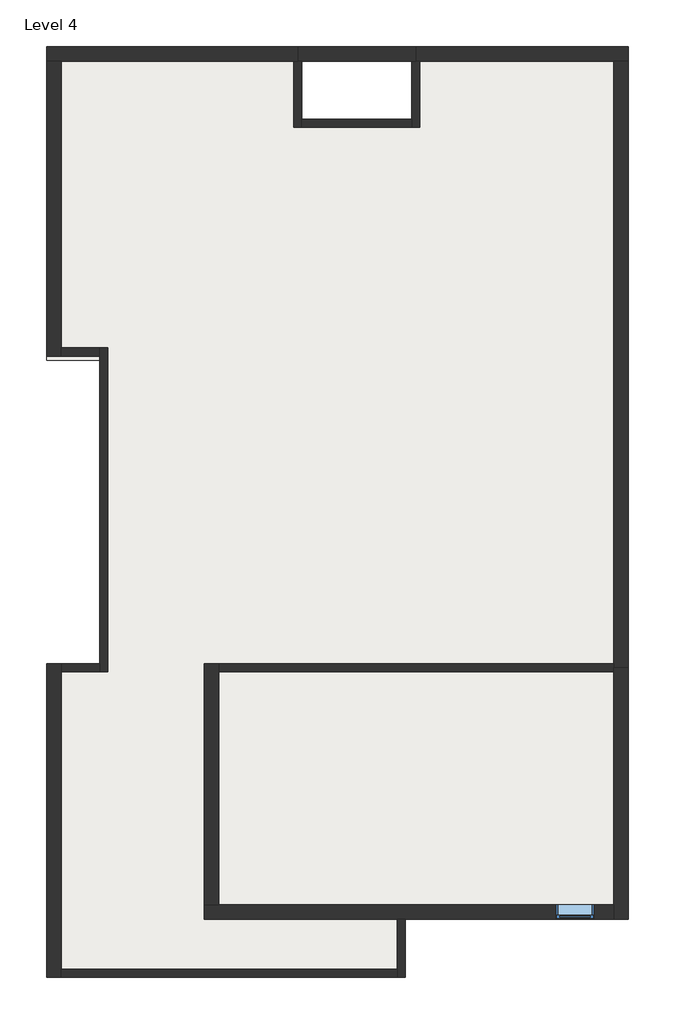
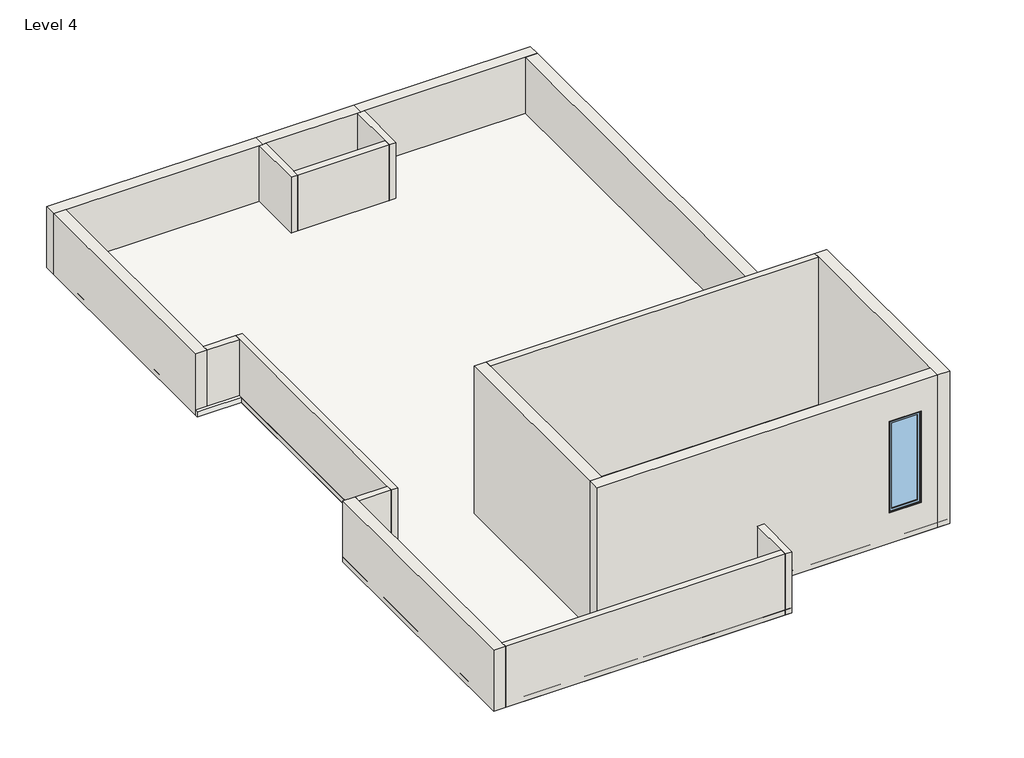
# One storey: 18 walls, 1 roof, 1 window.
"""IFC4 building model written with IfcOpenShell, lengths in millimetres."""

from ifc_helpers import new_model, si_unit, frame, origin, place, context, project, spatial, polyline, outline, extrude, faceted_brep, transform, mapped, element, save
from components import window_fc882ab3

model = new_model("IFC4")

# Units and contexts
model_context = context("Model", 3, world=origin())
ifc_project = project(units=[si_unit("LENGTHUNIT", "METRE", prefix="MILLI")], contexts=[model_context])

# Site, building, storey
site = spatial("IfcSite", under=ifc_project)
building = spatial("IfcBuilding", under=site)
storey = spatial("IfcBuildingStorey", under=building, Name="Level 4", Elevation=9144.0)

# Roof
placement = place(None, origin())
element("IfcRoof", 1, ObjectType="Generic - 4\"", at=placement, inside=storey, context=model_context, shape_type="Brep", body=[
    faceted_brep([(-5386.86646, 4170.6165298, 9144.0), (-5386.86646, 9098.2165298, 9144.0), (3757.13354, 9098.2165298, 9144.0), (3757.13354, -4617.7834702, 9144.0), (251.93354, -4617.7834702, 9144.0), (251.93354, -5532.1834702, 9144.0), (-5386.86646, -5532.1834702, 9144.0), (-5386.86646, -604.5834702, 9144.0), (-5158.26646, -604.5834702, 9144.0), (-4548.66646, -604.5834702, 9144.0), (-4548.66646, 4170.6165298, 9144.0), (-5158.26646, 4170.6165298, 9144.0), (353.53354, 8869.6165298, 9144.0), (-1373.66646, 8869.6165298, 9144.0), (-1373.66646, 7955.2165298, 9144.0), (353.53354, 7955.2165298, 9144.0), (3757.13354, -4617.7834702, 9245.6), (3757.13354, 9098.2165298, 9245.6), (-5386.86646, 9098.2165298, 9245.6), (-5386.86646, 4170.6165298, 9245.6), (-5158.26646, 4170.6165298, 9245.6), (-4548.66646, 4170.6165298, 9245.6), (-4548.66646, -604.5834702, 9245.6), (-5158.26646, -604.5834702, 9245.6), (-5386.86646, -604.5834702, 9245.6), (-5386.86646, -5532.1834702, 9245.6), (251.93354, -5532.1834702, 9245.6), (251.93354, -4617.7834702, 9245.6), (-1373.66646, 8869.6165298, 9245.6), (353.53354, 8869.6165298, 9245.6), (353.53354, 7955.2165298, 9245.6), (-1373.66646, 7955.2165298, 9245.6)], [[[0, 1, 2, 3, 4, 5, 6, 7, 8, 9, 10, 11], [12, 13, 14, 15]], [[16, 17, 18, 19, 20, 21, 22, 23, 24, 25, 26, 27], [28, 29, 30, 31]], [[2, 1, 18, 17]], [[1, 0, 19, 18]], [[3, 2, 17, 16]], [[4, 3, 16, 27]], [[5, 4, 27, 26]], [[6, 5, 26, 25]], [[22, 9, 8, 7, 24, 23]], [[10, 9, 22, 21]], [[19, 0, 11, 10, 21, 20]], [[7, 6, 25, 24]], [[12, 29, 28, 13]], [[13, 28, 31, 14]], [[14, 31, 30, 15]], [[29, 12, 15, 30]]]),
])

# Walls
element("IfcWall", 2, ObjectType="Generic - 5\"", at=placement, inside=storey, context=model_context, shape_type="Brep", body=[
    faceted_brep([(-2681.76646, -731.5834702, 9144.0), (3528.53354, -731.5834702, 9144.0), (3528.53354, -731.5834702, 12192.0), (-2681.76646, -731.5834702, 12192.0), (-2681.76646, -604.5834702, 9144.0), (-2681.76646, -604.5834702, 12192.0), (3528.53354, -604.5834702, 12192.0), (3528.53354, -604.5834702, 10363.2), (3528.53354, -604.5834702, 9144.0), (3528.53354, -668.0834702, 9144.0)], [[[0, 1, 2, 3]], [[4, 5, 6, 7, 8]], [[1, 0, 4, 8, 9]], [[3, 2, 6, 5]], [[1, 9, 8, 7, 6, 2]], [[0, 3, 5, 4]]]),
])
element("IfcWall", 3, ObjectType="Generic - 5\"", at=placement, inside=storey, context=model_context, shape_type="Brep", body=[
    faceted_brep([(-1500.66646, 8869.6165298, 9144.0), (-1500.66646, 7828.2165298, 9144.0), (-1500.66646, 7828.2165298, 10363.2), (-1500.66646, 8869.6165298, 10363.2), (-1373.66646, 8869.6165298, 9144.0), (-1373.66646, 8869.6165298, 10363.2), (-1373.66646, 7955.2165298, 10363.2), (-1373.66646, 7828.2165298, 10363.2), (-1373.66646, 7828.2165298, 9144.0), (-1373.66646, 7955.2165298, 9144.0), (-1437.16646, 8869.6165298, 9144.0), (-1437.16646, 8869.6165298, 10363.2)], [[[0, 1, 2, 3]], [[4, 5, 6, 7, 8, 9]], [[1, 0, 10, 4, 9, 8]], [[3, 2, 7, 6, 5, 11]], [[2, 1, 8, 7]], [[0, 3, 11, 5, 4, 10]]]),
])
element("IfcWall", 4, ObjectType="Generic - 5\"", at=placement, inside=storey, context=model_context, shape_type="Brep", body=[
    faceted_brep([(353.53354, 8869.6165298, 9144.0), (353.53354, 7955.2165298, 9144.0), (353.53354, 7828.2165298, 9144.0), (353.53354, 7828.2165298, 10363.2), (353.53354, 7955.2165298, 10363.2), (353.53354, 8869.6165298, 10363.2), (480.53354, 8869.6165298, 9144.0), (480.53354, 8869.6165298, 10363.2), (480.53354, 7828.2165298, 10363.2), (480.53354, 7828.2165298, 9144.0), (417.03354, 8869.6165298, 9144.0), (417.03354, 8869.6165298, 10363.2)], [[[0, 1, 2, 3, 4, 5]], [[6, 7, 8, 9]], [[2, 1, 0, 10, 6, 9]], [[5, 4, 3, 8, 7, 11]], [[3, 2, 9, 8]], [[0, 5, 11, 7, 6, 10]]]),
])
element("IfcWall", 5, ObjectType="Generic - 5\"", at=placement, inside=storey, context=model_context, shape_type="SweptSolid", body=[
    extrude(outline(polyline([(-1373.66646, 7955.2165298), (353.53354, 7955.2165298), (353.53354, 7828.2165298), (-1373.66646, 7828.2165298), (-1373.66646, 7955.2165298)])), frame((0.0, 0.0, 9144.0), z_axis=(0.0, 0.0, 1.0), x_axis=(1.0, 0.0, 0.0)), (0.0, 0.0, 1.0), 1219.2),
])
element("IfcWall", 6, ObjectType="Generic - 5\"", at=placement, inside=storey, context=model_context, shape_type="Brep", body=[
    faceted_brep([(-4421.66646, -731.5834702, 9144.0), (-4421.66646, 4361.1165298, 9144.0), (-4421.66646, 4361.1165298, 10363.2), (-4421.66646, -731.5834702, 10363.2), (-4548.66646, -731.5834702, 9144.0), (-4548.66646, -731.5834702, 10363.2), (-4548.66646, -604.5834702, 10363.2), (-4548.66646, 4234.1165298, 10363.2), (-4548.66646, 4361.1165298, 10363.2), (-4548.66646, 4361.1165298, 9144.0), (-4548.66646, 4234.1165298, 9144.0), (-4548.66646, -604.5834702, 9144.0)], [[[0, 1, 2, 3]], [[4, 5, 6, 7, 8, 9, 10, 11]], [[1, 0, 4, 11, 10, 9]], [[3, 2, 8, 7, 6, 5]], [[2, 1, 9, 8]], [[0, 3, 5, 4]]]),
])
element("IfcWall", 7, ObjectType="Generic - 5\"", at=placement, inside=storey, context=model_context, shape_type="SweptSolid", body=[
    extrude(outline(polyline([(-5158.26646, 4361.1165298), (-4548.66646, 4361.1165298), (-4548.66646, 4234.1165298), (-5158.26646, 4234.1165298), (-5158.26646, 4361.1165298)])), frame((0.0, 0.0, 9144.0), z_axis=(0.0, 0.0, 1.0), x_axis=(1.0, 0.0, 0.0)), (0.0, 0.0, 1.0), 1219.2),
])
element("IfcWall", 8, ObjectType="Generic - 5\"", at=placement, inside=storey, context=model_context, shape_type="SweptSolid", body=[
    extrude(outline(polyline([(-5158.26646, -604.5834702), (-4548.66646, -604.5834702), (-4548.66646, -731.5834702), (-5158.26646, -731.5834702), (-5158.26646, -604.5834702)])), frame((0.0, 0.0, 9144.0), z_axis=(0.0, 0.0, 1.0), x_axis=(1.0, 0.0, 0.0)), (0.0, 0.0, 1.0), 1219.2),
])
element("IfcWall", 9, ObjectType="Generic - 5\"", at=placement, inside=storey, context=model_context, shape_type="Brep", body=[
    faceted_brep([(124.93354, -4617.7834702, 9144.0), (124.93354, -5405.1834702, 9144.0), (124.93354, -5532.1834702, 9144.0), (124.93354, -5532.1834702, 10363.2), (124.93354, -5405.1834702, 10363.2), (124.93354, -4617.7834702, 10363.2), (251.93354, -4617.7834702, 9144.0), (251.93354, -4617.7834702, 10363.2), (251.93354, -5532.1834702, 10363.2), (251.93354, -5532.1834702, 9144.0)], [[[0, 1, 2, 3, 4, 5]], [[6, 7, 8, 9]], [[2, 1, 0, 6, 9]], [[5, 4, 3, 8, 7]], [[0, 5, 7, 6]], [[3, 2, 9, 8]]]),
])
element("IfcWall", 10, ObjectType="Generic - 5\"", at=placement, inside=storey, context=model_context, shape_type="SweptSolid", body=[
    extrude(outline(polyline([(-5158.26646, -5405.1834702), (124.93354, -5405.1834702), (124.93354, -5532.1834702), (-5158.26646, -5532.1834702), (-5158.26646, -5405.1834702)])), frame((0.0, 0.0, 9144.0), z_axis=(0.0, 0.0, 1.0), x_axis=(1.0, 0.0, 0.0)), (0.0, 0.0, 1.0), 1219.2),
])
element("IfcWall", 11, ObjectType="Generic -9\"", at=placement, inside=storey, context=model_context, shape_type="Brep", body=[
    faceted_brep([(-5386.86646, 8869.6165298, 9144.0), (-5158.26646, 8869.6165298, 9144.0), (-1500.66646, 8869.6165298, 9144.0), (-1437.16646, 8869.6165298, 9144.0), (-1437.16646, 8869.6165298, 10363.2), (-1500.66646, 8869.6165298, 10363.2), (-5158.26646, 8869.6165298, 10363.2), (-5386.86646, 8869.6165298, 10363.2), (-5386.86646, 9098.2165298, 9144.0), (-5386.86646, 9098.2165298, 10363.2), (-1437.16646, 9098.2165298, 10363.2), (-1437.16646, 9098.2165298, 9144.0)], [[[0, 1, 2, 3, 4, 5, 6, 7]], [[8, 9, 10, 11]], [[3, 2, 1, 0, 8, 11]], [[4, 3, 11, 10]], [[7, 6, 5, 4, 10, 9]], [[0, 7, 9, 8]]]),
])
element("IfcWall", 12, ObjectType="Generic -9\"", at=placement, inside=storey, context=model_context, shape_type="Brep", body=[
    faceted_brep([(3528.53354, 8869.6165298, 9144.0), (3528.53354, -604.5834702, 9144.0), (3528.53354, -668.0834702, 9144.0), (3528.53354, -668.0834702, 10363.2), (3528.53354, -604.5834702, 10363.2), (3528.53354, 8869.6165298, 10363.2), (3757.13354, 8869.6165298, 9144.0), (3757.13354, 8869.6165298, 10363.2), (3757.13354, -604.5834702, 10363.2), (3757.13354, -668.0834702, 10363.2), (3757.13354, -668.0834702, 9144.0)], [[[0, 1, 2, 3, 4, 5]], [[6, 7, 8, 9, 10]], [[2, 1, 0, 6, 10]], [[3, 2, 10, 9]], [[5, 4, 3, 9, 8, 7]], [[0, 5, 7, 6]]]),
])
element("IfcWall", 13, ObjectType="Generic -9\"", at=placement, inside=storey, context=model_context, shape_type="Brep", body=[
    faceted_brep([(3528.53354, -4389.1834702, 9144.0), (-2681.76646, -4389.1834702, 9144.0), (-2910.36646, -4389.1834702, 9144.0), (-2910.36646, -4389.1834702, 12192.0), (-2681.76646, -4389.1834702, 12192.0), (3528.53354, -4389.1834702, 12192.0), (2614.13354, -4389.1834702, 11582.4), (2614.13354, -4389.1834702, 9753.6), (3223.73354, -4389.1834702, 9753.6), (3223.73354, -4389.1834702, 11582.4), (3528.53354, -4617.7834702, 9144.0), (3528.53354, -4617.7834702, 12192.0), (-2910.36646, -4617.7834702, 12192.0), (-2910.36646, -4617.7834702, 9144.0), (124.93354, -4617.7834702, 9144.0), (251.93354, -4617.7834702, 9144.0), (2614.13354, -4617.7834702, 11582.4), (3223.73354, -4617.7834702, 11582.4), (3223.73354, -4617.7834702, 9753.6), (2614.13354, -4617.7834702, 9753.6)], [[[0, 1, 2, 3, 4, 5], [6, 7, 8, 9]], [[10, 11, 12, 13, 14, 15], [16, 17, 18, 19]], [[2, 1, 0, 10, 15, 14, 13]], [[5, 4, 3, 12, 11]], [[0, 5, 11, 10]], [[3, 2, 13, 12]], [[7, 6, 16, 19]], [[8, 7, 19, 18]], [[9, 8, 18, 17]], [[6, 9, 17, 16]]]),
])
element("IfcWall", 14, ObjectType="Generic -9\"", at=placement, inside=storey, context=model_context, shape_type="Brep", body=[
    faceted_brep([(-5158.26646, -5532.1834702, 9144.0), (-5158.26646, -5405.1834702, 9144.0), (-5158.26646, -731.5834702, 9144.0), (-5158.26646, -604.5834702, 9144.0), (-5158.26646, -604.5834702, 10363.2), (-5158.26646, -731.5834702, 10363.2), (-5158.26646, -5405.1834702, 10363.2), (-5158.26646, -5532.1834702, 10363.2), (-5386.86646, -5532.1834702, 9144.0), (-5386.86646, -5532.1834702, 10363.2), (-5386.86646, -604.5834702, 10363.2), (-5386.86646, -604.5834702, 9144.0)], [[[0, 1, 2, 3, 4, 5, 6, 7]], [[8, 9, 10, 11]], [[3, 2, 1, 0, 8, 11]], [[7, 6, 5, 4, 10, 9]], [[4, 3, 11, 10]], [[0, 7, 9, 8]]]),
])
element("IfcWall", 15, ObjectType="Generic -9\"", at=placement, inside=storey, context=model_context, shape_type="Brep", body=[
    faceted_brep([(-5158.26646, 4234.1165298, 9144.0), (-5158.26646, 4361.1165298, 9144.0), (-5158.26646, 8869.6165298, 9144.0), (-5158.26646, 8869.6165298, 10363.2), (-5158.26646, 4361.1165298, 10363.2), (-5158.26646, 4234.1165298, 10363.2), (-5386.86646, 4234.1165298, 9144.0), (-5386.86646, 4234.1165298, 10363.2), (-5386.86646, 8869.6165298, 10363.2), (-5386.86646, 8869.6165298, 9144.0)], [[[0, 1, 2, 3, 4, 5]], [[6, 7, 8, 9]], [[2, 1, 0, 6, 9]], [[5, 4, 3, 8, 7]], [[3, 2, 9, 8]], [[0, 5, 7, 6]]]),
])
element("IfcWall", 16, ObjectType="Generic -9\"", at=placement, inside=storey, context=model_context, shape_type="Brep", body=[
    faceted_brep([(3528.53354, -668.0834702, 9144.0), (3528.53354, -731.5834702, 9144.0), (3528.53354, -4389.1834702, 9144.0), (3528.53354, -4617.7834702, 9144.0), (3528.53354, -4617.7834702, 12192.0), (3528.53354, -4389.1834702, 12192.0), (3528.53354, -731.5834702, 12192.0), (3528.53354, -604.5834702, 12192.0), (3528.53354, -604.5834702, 10363.2), (3528.53354, -668.0834702, 10363.2), (3757.13354, -668.0834702, 9144.0), (3757.13354, -668.0834702, 10363.2), (3757.13354, -604.5834702, 10363.2), (3757.13354, -604.5834702, 12192.0), (3757.13354, -4617.7834702, 12192.0), (3757.13354, -4617.7834702, 9144.0)], [[[0, 1, 2, 3, 4, 5, 6, 7, 8, 9]], [[10, 11, 12, 13, 14, 15]], [[3, 2, 1, 0, 10, 15]], [[7, 6, 5, 4, 14, 13]], [[4, 3, 15, 14]], [[0, 9, 11, 10]], [[8, 12, 11, 9]], [[8, 7, 13, 12]]]),
])
element("IfcWall", 17, ObjectType="Generic -9\"", at=placement, inside=storey, context=model_context, shape_type="Brep", body=[
    faceted_brep([(417.03354, 8869.6165298, 9144.0), (480.53354, 8869.6165298, 9144.0), (3528.53354, 8869.6165298, 9144.0), (3757.13354, 8869.6165298, 9144.0), (3757.13354, 8869.6165298, 10363.2), (3528.53354, 8869.6165298, 10363.2), (480.53354, 8869.6165298, 10363.2), (417.03354, 8869.6165298, 10363.2), (417.03354, 9098.2165298, 9144.0), (417.03354, 9098.2165298, 10363.2), (3757.13354, 9098.2165298, 10363.2), (3757.13354, 9098.2165298, 9144.0)], [[[0, 1, 2, 3, 4, 5, 6, 7]], [[8, 9, 10, 11]], [[3, 2, 1, 0, 8, 11]], [[7, 6, 5, 4, 10, 9]], [[0, 7, 9, 8]], [[4, 3, 11, 10]]]),
])
element("IfcWall", 18, ObjectType="Generic -9\"", at=placement, inside=storey, context=model_context, shape_type="Brep", body=[
    faceted_brep([(-1437.16646, 8869.6165298, 9144.0), (-1373.66646, 8869.6165298, 9144.0), (353.53354, 8869.6165298, 9144.0), (417.03354, 8869.6165298, 9144.0), (417.03354, 8869.6165298, 10363.2), (353.53354, 8869.6165298, 10363.2), (-1373.66646, 8869.6165298, 10363.2), (-1437.16646, 8869.6165298, 10363.2), (-1437.16646, 9098.2165298, 9144.0), (-1437.16646, 9098.2165298, 10363.2), (417.03354, 9098.2165298, 10363.2), (417.03354, 9098.2165298, 9144.0)], [[[0, 1, 2, 3, 4, 5, 6, 7]], [[8, 9, 10, 11]], [[3, 2, 1, 0, 8, 11]], [[4, 3, 11, 10]], [[7, 6, 5, 4, 10, 9]], [[0, 7, 9, 8]]]),
])
element("IfcWall", 19, ObjectType="Generic -9\"", at=placement, inside=storey, context=model_context, shape_type="Brep", body=[
    faceted_brep([(-2681.76646, -4389.1834702, 9144.0), (-2681.76646, -731.5834702, 9144.0), (-2681.76646, -604.5834702, 9144.0), (-2681.76646, -604.5834702, 12192.0), (-2681.76646, -731.5834702, 12192.0), (-2681.76646, -4389.1834702, 12192.0), (-2910.36646, -4389.1834702, 9144.0), (-2910.36646, -4389.1834702, 12192.0), (-2910.36646, -604.5834702, 12192.0), (-2910.36646, -604.5834702, 9144.0)], [[[0, 1, 2, 3, 4, 5]], [[6, 7, 8, 9]], [[2, 1, 0, 6, 9]], [[5, 4, 3, 8, 7]], [[0, 5, 7, 6]], [[3, 2, 9, 8]]]),
])

# Window
window_shape = window_fc882ab3(model_context)
element("IfcWindow", 20, ObjectType="Fixed : 24\" x 72\"", at=placement, inside=storey, context=model_context, shape_type="MappedRepresentation", body=[
    mapped(window_shape, transform((2880.83354, -4503.4834702, 9448.8), x_axis=(-1.0, 0.0, 0.0), y_axis=(0.0, -1.0, 0.0), z_axis=(0.0, 0.0, 1.0))),
])

save(model, "model.ifc")

# Revit data of these elements
# Type "Generic - 4\""
#   Assembly Code = "B1020"
#   Layers, outside or top first: 0' - 4" no material (function 1)
# Type "Generic - 5\""
#   Assembly Code = "B2010"
#   Layers, outside or top first: 0' - 5" no material (function 1)
# Type "Generic -9\""
#   Assembly Code = "B2010"
#   Layers, outside or top first: 0' - 9" no material (function 1)
# Type "Fixed : 24\" x 72\""
#   Type Mark = "7"
#   Assembly Code = "B2020100"
#   Height = 6' - 0"
#   Default Sill Height = 1' - 0"
#   Width = 2' - 0"
#   Window Inset = 0' - 0 3/4"
#   Glass Pane Material = Glass
#   Sash Material = Sash
#   Wall Closure = (empty or 0)
# Element 1 (IfcRoof, "Generic - 4\"")
#   built-in parameter 1001705 = 30.3333 (stored number, unit not read)
#   built-in parameter 1001710 = 33615
#   Phase Created = New Construction
#   Materials on its faces: "Default Roof"
# Element 2 (IfcWall, "Generic - 5\"")
#   Top Offset = 0' - 0"
#   Base Offset = 0' - 0"
#   Unconnected Height = 10' - 0"
#   wall height = 10' - 0"
#   Phase Created = New Construction
#   Base Constraint = Level 4
#   Materials on its faces: "Default Wall"
# Elements 3, 4, 5, 6, 7, 8, 9, 10 (IfcWall, "Generic - 5\"")
#   Top Offset = 0' - 0"
#   Base Offset = 0' - 0"
#   Unconnected Height = 4' - 0"
#   wall height = 4' - 0"
#   Phase Created = New Construction
#   Base Constraint = Level 4
#   Materials on its faces: "Default Wall"
# Elements 11, 12, 14, 15, 17, 18 (IfcWall, "Generic -9\"")
#   Top Offset = 0' - 0"
#   Base Offset = 0' - 0"
#   Unconnected Height = 4' - 0"
#   wall height = 4' - 0"
#   Phase Created = New Construction
#   Base Constraint = Level 4
#   Materials on its faces: "Default Wall"
# Elements 13, 16 (IfcWall, "Generic -9\"")
#   Top Offset = 0' - 0"
#   Base Offset = 0' - 0"
#   Unconnected Height = 10' - 0"
#   wall height = 10' - 0"
#   Phase Created = New Construction
#   Base Constraint = Level 4
#   Materials on its faces: "Default Wall", "01 colour"
# Element 19 (IfcWall, "Generic -9\"")
#   Top Offset = 0' - 0"
#   Base Offset = 0' - 0"
#   Unconnected Height = 10' - 0"
#   wall height = 10' - 0"
#   Phase Created = New Construction
#   Base Constraint = Level 4
#   Materials on its faces: "Default Wall"
# Element 20 (IfcWindow, "Fixed : 24\" x 72\"")
#   Mark = "4"
#   Phase Created = New Construction
#   Materials on its faces: "Sash", "Glass"
# Materials
#   "Glass": class "Glass", colour RGB 218 227 224, transparency 0.85, Description = "Soda Lime Glass", Cost = 0
#   "Sash": class "Wood", colour RGB 136 99 55, transparency 0
#   "Default Roof": colour RGB 80 80 80, transparency 0
#   "Default Wall": colour RGB 80 80 80, transparency 0
#   "01 colour": class "Generic", colour RGB 120 120 120, transparency 0, Cost = 0
